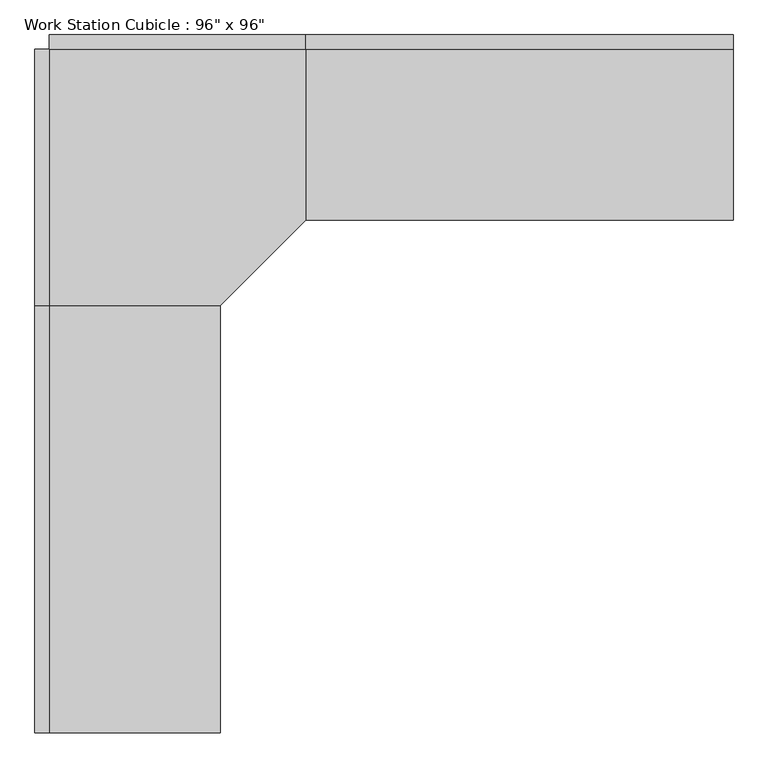
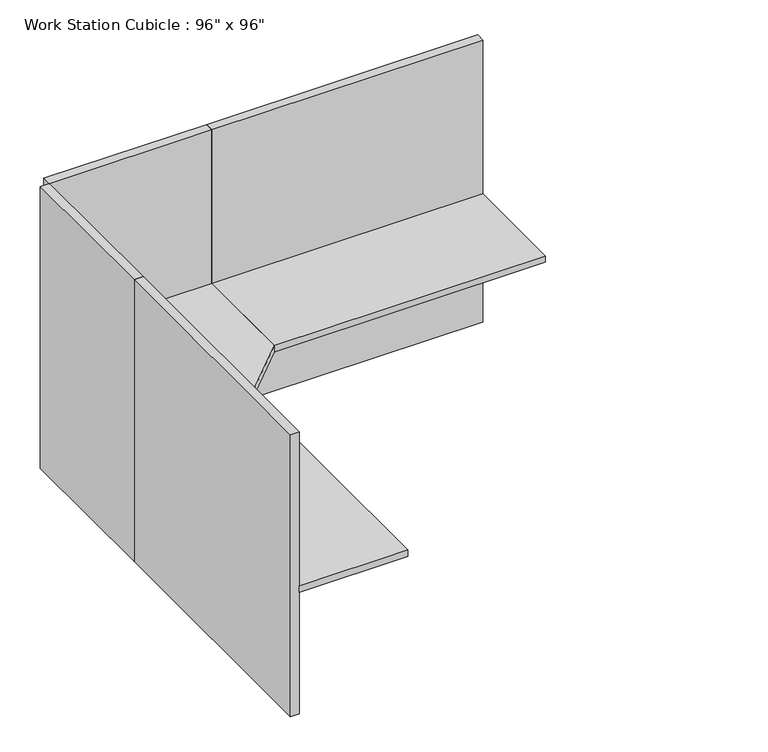
"""IFC4 building model written with IfcOpenShell, lengths in millimetres: furniture geometry."""

from ifc_helpers import new_model, si_unit, frame, origin, origin_with_axes, place, context, project, spatial, polyline, outline, extrude, source, transform, mapped, element, save


def furniture_45e3acac(model_context):
    return source(origin(), model_context, "Body", "SweptSolid", [
        extrude(outline(polyline([(-80.9317522, -545.8230076), (833.4682478, -545.8230076), (833.4682478, -1155.4230076), (528.6682478, -1460.2230076), (-80.9317522, -1460.2230076), (-80.9317522, -545.8230076)])), frame((0.0, 0.0, 723.9), z_axis=(0.0, 0.0, 1.0), x_axis=(1.0, 0.0, 0.0)), (0.0, 0.0, 1.0), 38.1),
        extrude(outline(polyline([(528.6682478, -2984.2230076), (-80.9317522, -2984.2230076), (-80.9317522, -1460.2230076), (528.6682478, -1460.2230076), (528.6682478, -2984.2230076)])), frame((0.0, 0.0, 723.9), z_axis=(0.0, 0.0, 1.0), x_axis=(1.0, 0.0, 0.0)), (0.0, 0.0, 1.0), 38.1),
        extrude(outline(polyline([(2357.4682478, -1155.4230076), (833.4682478, -1155.4230076), (833.4682478, -545.8230076), (2357.4682478, -545.8230076), (2357.4682478, -1155.4230076)])), frame((0.0, 0.0, 723.9), z_axis=(0.0, 0.0, 1.0), x_axis=(1.0, 0.0, 0.0)), (0.0, 0.0, 1.0), 38.1),
        extrude(outline(polyline([(2357.4682478, -545.8230076), (833.4682478, -545.8230076), (833.4682478, -495.0230076), (2357.4682478, -495.0230076), (2357.4682478, -545.8230076)])), origin_with_axes(), (0.0, 0.0, 1.0), 1676.4),
        extrude(outline(polyline([(833.4682478, -545.8230076), (-80.9317522, -545.8230076), (-80.9317522, -495.0230076), (833.4682478, -495.0230076), (833.4682478, -545.8230076)])), origin_with_axes(), (0.0, 0.0, 1.0), 1676.4),
        extrude(outline(polyline([(-80.9317522, -1460.2230076), (-131.7317522, -1460.2230076), (-131.7317522, -545.8230076), (-80.9317522, -545.8230076), (-80.9317522, -1460.2230076)])), origin_with_axes(), (0.0, 0.0, 1.0), 1676.4),
        extrude(outline(polyline([(-80.9317522, -2984.2230076), (-131.7317522, -2984.2230076), (-131.7317522, -1460.2230076), (-80.9317522, -1460.2230076), (-80.9317522, -2984.2230076)])), origin_with_axes(), (0.0, 0.0, 1.0), 1676.4),
    ])


if __name__ == "__main__":
    model = new_model("IFC4")
    model_context = context("Model", 3, world=origin())
    ifc_project = project(units=[si_unit("LENGTHUNIT", "METRE", prefix="MILLI")], contexts=[model_context])
    site = spatial("IfcSite", under=ifc_project)
    building = spatial("IfcBuilding", under=site)
    placement = place(None, origin())
    furniture_shape = furniture_45e3acac(model_context)
    element("IfcFurniture", 1, ObjectType="Work Station Cubicle : 96\" x 96\"", at=placement, inside=building, context=model_context, shape_type="MappedRepresentation", body=[
        mapped(furniture_shape, transform((0.0, 0.0, 0.0), x_axis=(1.0, 0.0, 0.0), y_axis=(0.0, 1.0, 0.0), z_axis=(0.0, 0.0, 1.0))),
    ])
    save(model, "model.ifc")

# Revit data of these elements
# Type "Work Station Cubicle : 96\" x 96\""
#   Assembly Code = "E2020"
#   Desktop Height = 2' - 6"
#   Desktop1 Width = 2' - 0"
#   Desktop2 Width = 2' - 0"
#   Panel Height = 5' - 6"
#   Panel1 Length = 5' - 0"
#   Panel2 Length = 5' - 0"
#   Cube Panel Material = Textile - Light Gray
#   Work Top Material = Laminate, Ivory, Matte
#   Default Elevation = 0
# Element 1 (IfcFurniture, "Work Station Cubicle : 96\" x 96\"")
#   Materials on its faces: "Textile - Light Gray", "Laminate, Ivory, Matte"
# Materials
#   "Textile - Light Gray": class "Fabric", colour RGB 204 204 204, transparency 0
#   "Laminate, Ivory, Matte": class "Plastic", colour RGB 247 247 239, transparency 0, Description = "Plastic Laminate - Ivory, Matte", Cost = 0
